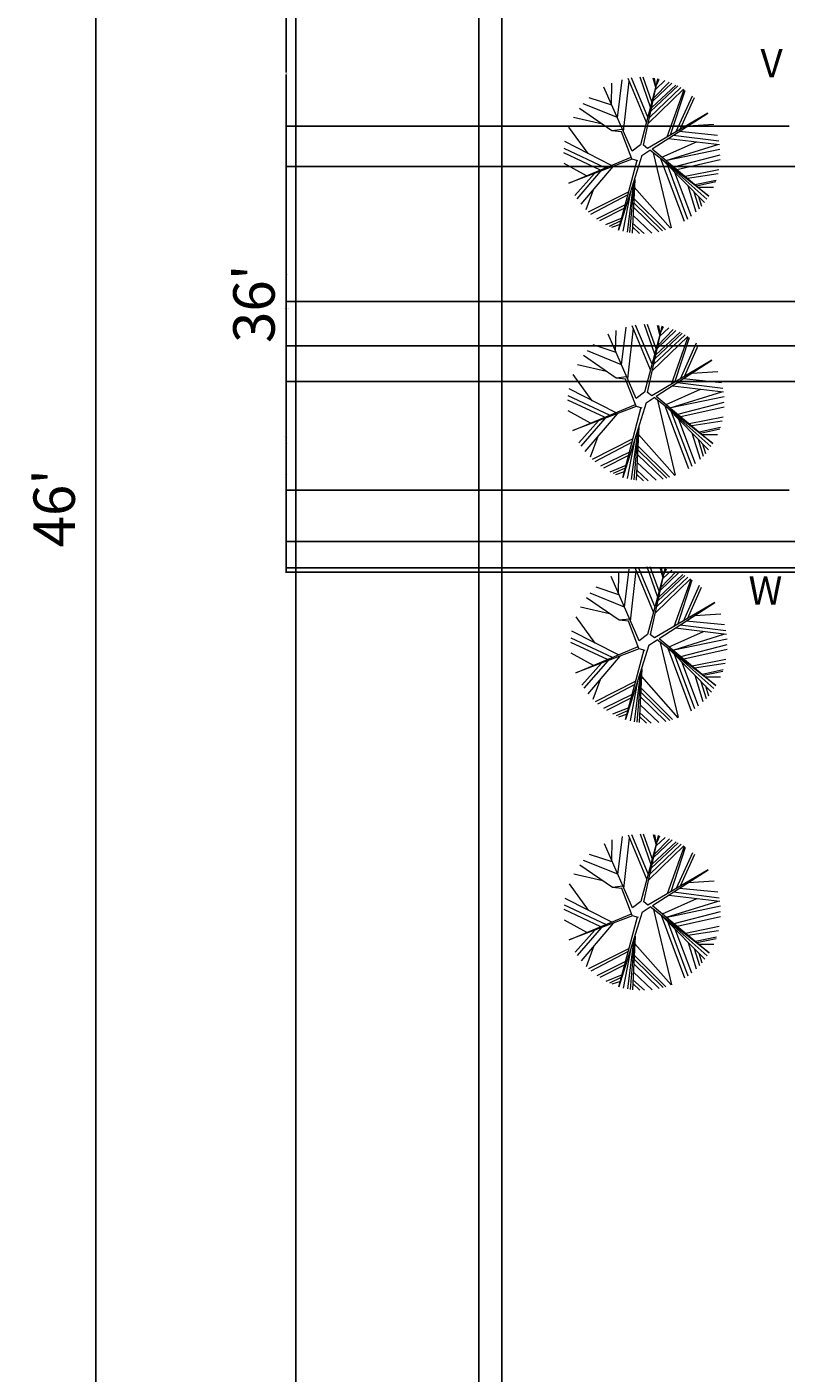
# Model space of a CAD drawing. Units: inches. Extents: x 503 to 1084, y -605 to 132.
# Tile 2 of 14: x 503 to 649, y -437 to -177. Entities that reach past the tile are written whole.
import ezdxf

# ---------------------------------------------------------------- set-up
doc = ezdxf.new("R2010")
doc.units = ezdxf.units.IN
doc.header["$MEASUREMENT"] = 0
for name, color, linetype, lineweight in [('A-ANNO-DIMS', 7, 'Continuous', 18), ('A-ANNO-TEXT', 7, 'Continuous', 18), ('C-PROP', 1, 'Continuous', 25)]:
    doc.layers.add(name, color=color, linetype=linetype, lineweight=lineweight)
doc.layers.add('GRASS', color=90, linetype='Continuous', lineweight=13, transparency=0.7)
doc.styles.get("Standard").update_dxf_attribs({"font": 'arial.ttf'})
doc.dimstyles.get("Standard").update_dxf_attribs({"dimtxt": 0.18, "dimasz": 0.18, "dimexe": 0.18, "dimexo": 0.0625, "dimgap": 0.09, "dimtad": 0, "dimtih": 1, "dimtoh": 1, "dimdec": 1, "dimzin": 0, "dimdsep": 46, "dimlunit": 4, "dimtxsty": 'Standard', "dimcen": 0.09, "dimadec": 0, "dimazin": 0, "dimtfac": 1, "dimtdec": 1, "dimtofl": 0, "dimtmove": 0, "dimatfit": 3, "dimfxl": 1, "dimtolj": 1, "dimtzin": 0, "dimarcsym": 0})

# ---------------------------------------------------------------- blocks, each defined once
blk = doc.blocks.new('A$C4FA53466')
at = {"color": 0}
for p, q in [((0.501, 1.356), (0.505, 1.578)), ((0.563, 1.216), (0.612, 1.614)), ((0.627, 1.07), (0.687, 1.601)), ((0.867, 1.166), (0.675, 1.628)), ((0.882, 1.223), (0.709, 1.633)), ((0.91, 1.328), (0.802, 1.64)), ((0.988, 1.623), (0.804, 0.931)), ((0.925, 1.384), (0.834, 1.64)), ((0.836, 0.927), (0.988, 1.623)), ((0.922, 1.323), (1.176, 1.559)), ((0.964, 1.534), (0.938, 1.632)), ((0.938, 1.393), (1.132, 1.579)), ((0.945, 1.425), (1.104, 1.59)), ((0.967, 1.545), (0.952, 1.63)), ((0.965, 1.517), (1.059, 1.605)), ((0.974, 1.559), (1.002, 1.62)), ((0.505, 1.347), (0.266, 1.426)), ((0.717, 0.864), (0.422, 1.538)), ((0.887, 1.159), (1.256, 1.515)), ((0.901, 1.223), (1.228, 1.532)), ((0.914, 1.283), (1.197, 1.549)), ((1.085, 1.015), (1.262, 1.512)), ((1.121, 1.036), (1.274, 1.503)), ((1.18, 1.071), (1.349, 1.447)), ((1.222, 1.096), (1.37, 1.428)), ((0.506, 1.079), (0.165, 1.314)), ((0.562, 1.217), (0.205, 1.363)), ((0.406, 1.148), (0.102, 1.217)), ((1.509, 1.265), (0.879, 0.894)), ((0.926, 0.889), (1.509, 1.265)), ((1.3, 1.13), (1.573, 1.147)), ((0.255, 0.841), (0.055, 1.116)), ((0.614, 1.092), (0.506, 1.079)), ((0.604, 1.069), (0.506, 1.079)), ((0.715, 0.784), (0.604, 1.069)), ((1.097, 0.999), (1.632, 0.934)), ((1.148, 1.032), (1.626, 0.972)), ((1.211, 1.073), (1.612, 1.034)), ((0.384, 0.667), (0, 0.848)), ((0.436, 0.689), (0.003, 0.892)), ((0.501, 0.716), (0.012, 0.965)), ((0.804, 0.931), (0.717, 0.864)), ((0.82, 0.82), (0.904, 0.875)), ((0.879, 0.894), (0.836, 0.927)), ((1.521, 0.394), (0.904, 0.875)), ((0.926, 0.889), (1.521, 0.394)), ((0.938, 0.848), (1.126, 0.059)), ((1.03, 0.802), (1.392, 0.963)), ((1.073, 0.767), (1.614, 0.936)), ((1.081, 0.769), (1.638, 0.886)), ((0.237, 0.605), (0.004, 0.735)), ((0.053, 0.528), (0.708, 0.803)), ((0.716, 0.781), (0.053, 0.528)), ((0.82, 0.82), (0.575, 0.037)), ((0.575, 0.037), (0.769, 0.772)), ((0.715, 0.784), (0.775, 0.767)), ((1.016, 0.788), (1.263, 0.13)), ((1.04, 0.769), (1.475, 0.326)), ((1.06, 0.754), (1.5, 0.362)), ((1.083, 0.725), (1.298, 0.153)), ((1.153, 0.701), (1.64, 0.826)), ((1.185, 0.674), (1.639, 0.776)), ((0.321, 0.63), (0.115, 0.4)), ((0.387, 0.655), (0.137, 0.366)), ((0.516, 0.704), (0.179, 0.309)), ((0.744, 0.569), (0.717, 0.006)), ((1.161, 0.646), (1.335, 0.182)), ((1.273, 0.601), (1.627, 0.672)), ((1.298, 0.58), (1.618, 0.629)), ((0.313, 0.466), (0.232, 0.248)), ((0.682, 0.44), (0.255, 0.225)), ((0.701, 0.44), (0.621, 0.024)), ((0.732, 0.539), (0.664, 0.015)), ((0.737, 0.554), (0.691, 0.01)), ((0.74, 0.488), (1.121, 0.057)), ((1.301, 0.503), (1.386, 0.227)), ((1.365, 0.438), (1.42, 0.26)), ((1.376, 0.515), (1.599, 0.562)), ((1.392, 0.502), (1.593, 0.545)), ((1.412, 0.486), (1.569, 0.486)), ((0.673, 0.407), (0.281, 0.201)), ((0.645, 0.301), (0.342, 0.153)), ((0.733, 0.326), (1.037, 0.029)), ((0.735, 0.369), (1.067, 0.038)), ((1.413, 0.39), (1.444, 0.288)), ((0.636, 0.267), (0.375, 0.133)), ((0.608, 0.161), (0.439, 0.093)), ((0.726, 0.192), (0.924, 0.006)), ((0.73, 0.277), (0.998, 0.019)), ((0.6, 0.133), (0.475, 0.076)), ((0.59, 0.094), (0.501, 0.064)), ((0.72, 0.07), (0.793, 0)), ((0.722, 0.111), (0.842, 0))]:
    blk.add_line(p, q, dxfattribs=at)
blk = doc.blocks.new('_ArchTick')
at = {"color": 0, "linetype": 'ByBlock', "const_width": 0.15}
blk.add_lwpolyline([(-0.5, -0.5), (0.5, 0.5)], dxfattribs=at)
blk = doc.blocks.new('_Oblique')
at = {"color": 0, "linetype": 'ByBlock', "lineweight": -2}
blk.add_line((-0.5, -0.5), (0.5, 0.5), dxfattribs=at)
blk = doc.blocks.new('*D10')
at = {"layer": 'A-ANNO-DIMS', "color": 0, "lineweight": -2, "transparency": 16777216}
blk.add_line((516.2, 6.18), (516.2, -545.82), dxfattribs=at)
at = {"layer": 'Defpoints', "color": 0, "transparency": 16777216}
for p in [(590.09, 6.18), (516.2, -545.82), (590.09, -545.82)]:
    blk.add_point(p, dxfattribs=at)
at = {"layer": 'A-ANNO-DIMS', "color": 0, "lineweight": -2, "transparency": 16777216, "xscale": 5, "yscale": 5, "zscale": 5}
for name, p, rotation in [('_ArchTick', (516.2, 6.18), 90), ('_Oblique', (516.2, -545.82), 270)]:
    blk.add_blockref(name, p, dxfattribs=dict(at, rotation=rotation))
at = {"layer": 'A-ANNO-DIMS', "color": 0, "transparency": 16777216, "insert": (508.12, -269.82), "char_height": 8, "attachment_point": 5, "rotation": 90}
blk.add_mtext("\\A1;46'", dxfattribs=at)
blk = doc.blocks.new('*D12')
at = {"layer": 'A-ANNO-DIMS', "color": 0, "lineweight": -2, "transparency": 16777216}
blk.add_line((554.79, -17.82), (554.79, -442.82), dxfattribs=at)
at = {"layer": 'Defpoints', "color": 0, "transparency": 16777216}
for p in [(650.09, -17.82), (554.79, -442.82), (650.09, -442.82)]:
    blk.add_point(p, dxfattribs=at)
at = {"layer": 'A-ANNO-DIMS', "color": 0, "lineweight": -2, "transparency": 16777216, "xscale": 5, "yscale": 5, "zscale": 5}
for name, p, rotation in [('_ArchTick', (554.79, -17.82), 90), ('_Oblique', (554.79, -442.82), 270)]:
    blk.add_blockref(name, p, dxfattribs=dict(at, rotation=rotation))
at = {"layer": 'A-ANNO-DIMS', "color": 0, "transparency": 16777216, "insert": (546.7, -230.32), "char_height": 8, "attachment_point": 5, "rotation": 90}
blk.add_mtext("\\A1;36'", dxfattribs=at)
blk = doc.blocks.new('*D54')
at = {"layer": 'A-ANNO-DIMS', "color": 0, "lineweight": -2, "transparency": 16777216}
for p, q in [((650.03, -195.98), (552.76, -195.98)), ((552.94, -196.16), (552.94, -230.97)), ((552.94, -266.14), (552.94, -231.33)), ((650.03, -266.32), (552.76, -266.32))]:
    blk.add_line(p, q, dxfattribs=at)
at = {"layer": 'A-ANNO-DIMS', "color": 0, "transparency": 16777216}
for points in [[(552.91, -196.16), (552.97, -196.16), (552.94, -195.98)], [(552.91, -266.14), (552.97, -266.14), (552.94, -266.32)]]:
    blk.add_solid(points, dxfattribs=at)
at = {"layer": 'Defpoints', "color": 0, "transparency": 16777216}
for p in [(650.09, -195.98), (552.94, -266.32), (650.09, -266.32)]:
    blk.add_point(p, dxfattribs=at)
at = {"layer": 'A-ANNO-DIMS', "color": 0, "transparency": 16777216, "insert": (552.94, -231.15), "char_height": 0.18, "attachment_point": 5}
blk.add_mtext('\\A1;5\'-10 1/2"', dxfattribs=at)
blk = doc.blocks.new('*D55')
at = {"layer": 'A-ANNO-DIMS', "color": 0, "lineweight": -2, "transparency": 16777216}
for p, q in [((779.03, -245.32), (552.76, -245.32)), ((552.94, -245.5), (552.94, -263.13)), ((552.94, -281.14), (552.94, -263.5)), ((779.03, -281.32), (552.76, -281.32))]:
    blk.add_line(p, q, dxfattribs=at)
at = {"layer": 'A-ANNO-DIMS', "color": 0, "transparency": 16777216}
for points in [[(552.91, -245.5), (552.97, -245.5), (552.94, -245.32)], [(552.91, -281.14), (552.97, -281.14), (552.94, -281.32)]]:
    blk.add_solid(points, dxfattribs=at)
at = {"layer": 'Defpoints', "color": 0, "transparency": 16777216}
for p in [(779.09, -245.32), (552.94, -281.32), (779.09, -281.32)]:
    blk.add_point(p, dxfattribs=at)
at = {"layer": 'A-ANNO-DIMS', "color": 0, "transparency": 16777216, "insert": (552.94, -263.32), "char_height": 0.18, "attachment_point": 5}
blk.add_mtext('\\A1;3\'-0"', dxfattribs=at)
blk = doc.blocks.new('*D56')
at = {"layer": 'A-ANNO-DIMS', "color": 0, "lineweight": -2, "transparency": 16777216}
for p, q in [((779.03, -167.82), (552.76, -167.82)), ((552.94, -168), (552.94, -185.63)), ((552.94, -203.64), (552.94, -186)), ((779.03, -203.82), (552.76, -203.82))]:
    blk.add_line(p, q, dxfattribs=at)
at = {"layer": 'A-ANNO-DIMS', "color": 0, "transparency": 16777216}
for points in [[(552.91, -168), (552.97, -168), (552.94, -167.82)], [(552.91, -203.64), (552.97, -203.64), (552.94, -203.82)]]:
    blk.add_solid(points, dxfattribs=at)
at = {"layer": 'Defpoints', "color": 0, "transparency": 16777216}
for p in [(779.09, -167.82), (552.94, -203.82), (779.09, -203.82)]:
    blk.add_point(p, dxfattribs=at)
at = {"layer": 'A-ANNO-DIMS', "color": 0, "transparency": 16777216, "insert": (552.94, -185.82), "char_height": 0.18, "attachment_point": 5}
blk.add_mtext('\\A1;3\'-0"', dxfattribs=at)
blk = doc.blocks.new('*D62')
at = {"layer": 'A-ANNO-DIMS', "color": 0, "lineweight": -2, "transparency": 16777216}
for p, q in [((779.03, -203.82), (552.76, -203.82)), ((552.94, -204), (552.94, -224.38)), ((552.94, -245.14), (552.94, -224.75)), ((779.03, -245.32), (552.76, -245.32))]:
    blk.add_line(p, q, dxfattribs=at)
at = {"layer": 'A-ANNO-DIMS', "color": 0, "transparency": 16777216}
for points in [[(552.91, -204), (552.97, -204), (552.94, -203.82)], [(552.91, -245.14), (552.97, -245.14), (552.94, -245.32)]]:
    blk.add_solid(points, dxfattribs=at)
at = {"layer": 'Defpoints', "color": 0, "transparency": 16777216}
for p in [(779.09, -203.82), (552.94, -245.32), (779.09, -245.32)]:
    blk.add_point(p, dxfattribs=at)
at = {"layer": 'A-ANNO-DIMS', "color": 0, "transparency": 16777216, "insert": (552.94, -224.57), "char_height": 0.18, "attachment_point": 5}
blk.add_mtext('\\A1;3\'-5 1/2"', dxfattribs=at)
blk = doc.blocks.new('*D72')
at = {"layer": 'A-ANNO-DIMS', "color": 0, "lineweight": -2, "transparency": 16777216}
for p, q in [((948.89, -229.87), (552.76, -229.87)), ((552.94, -230.05), (552.94, -255.86)), ((552.94, -282.03), (552.94, -256.22)), ((949.25, -282.21), (552.76, -282.21))]:
    blk.add_line(p, q, dxfattribs=at)
at = {"layer": 'A-ANNO-DIMS', "color": 0, "transparency": 16777216}
for points in [[(552.91, -230.05), (552.97, -230.05), (552.94, -229.87)], [(552.91, -282.03), (552.97, -282.03), (552.94, -282.21)]]:
    blk.add_solid(points, dxfattribs=at)
at = {"layer": 'Defpoints', "color": 0, "transparency": 16777216}
for p in [(948.95, -229.87), (552.94, -282.21), (949.31, -282.21)]:
    blk.add_point(p, dxfattribs=at)
at = {"layer": 'A-ANNO-DIMS', "color": 0, "transparency": 16777216, "insert": (552.94, -256.04), "char_height": 0.18, "attachment_point": 5}
blk.add_mtext('\\A1;4\'-4 1/2"', dxfattribs=at)
blk = doc.blocks.new('*D77')
at = {"layer": 'A-ANNO-DIMS', "color": 0, "lineweight": -2, "transparency": 16777216}
for p, q in [((926.53, -238.47), (552.76, -238.47)), ((552.94, -238.65), (552.94, -257.17)), ((552.94, -276.07), (552.94, -257.54)), ((916.28, -276.25), (552.76, -276.25))]:
    blk.add_line(p, q, dxfattribs=at)
at = {"layer": 'A-ANNO-DIMS', "color": 0, "transparency": 16777216}
for points in [[(552.91, -238.65), (552.97, -238.65), (552.94, -238.47)], [(552.91, -276.07), (552.97, -276.07), (552.94, -276.25)]]:
    blk.add_solid(points, dxfattribs=at)
at = {"layer": 'Defpoints', "color": 0, "transparency": 16777216}
for p in [(926.59, -238.47), (552.94, -276.25), (916.35, -276.25)]:
    blk.add_point(p, dxfattribs=at)
at = {"layer": 'A-ANNO-DIMS', "color": 0, "transparency": 16777216, "insert": (552.94, -257.36), "char_height": 0.18, "attachment_point": 5}
blk.add_mtext('\\A1;3\'-2"', dxfattribs=at)

msp = doc.modelspace()

# ---------------------------------------------------------------- linework, layer by layer
at = {"layer": 'C-PROP'}
for p, q in [((590.09, 6.18), (590.09, -545.82)), ((594.59, -541.32), (594.59, 1.68))]:
    msp.add_line(p, q, dxfattribs=at)

# ---------------------------------------------------------------- block references
at = {"layer": 'GRASS', "xscale": 18.41745235960633, "yscale": 18.41745235960633, "zscale": 18.41745235960633}
for p in [(606.51, -216.77), (607.31, -264.55), (607.87, -311.36), (606.58, -362.98)]:
    msp.add_blockref('A$C4FA53466', p, dxfattribs=at)

# ---------------------------------------------------------------- texts
at = {"layer": 'A-ANNO-TEXT'}
for s, p in [('V', (644.51, -186.57)), ('W', (642.19, -288.44))]:
    msp.add_text(s, height=5.44, dxfattribs=at).set_placement(p)

# ---------------------------------------------------------------- dimensions: what is measured, and where the dimension line sits
at = {"layer": 'A-ANNO-DIMS'}
for base, p1, p2, override, picture, middle in [((516.2, -545.82), (590.09, 6.18), (590.09, -545.82), {"dimtxt": 8, "dimasz": 5, "dimgap": 4, "dimtad": 1, "dimtih": 0, "dimblk1": 'ArchTick', "dimblk2": 'Oblique', "dimsah": 1, "dimse1": 1, "dimse2": 1, "dimclrd": 0, "dimclre": 0, "dimclrt": 0}, '*D10', (508.12, -269.82)), ((552.94, -203.82), (779.09, -167.82), (779.09, -203.82), {"dimdec": 1, "dimlfac": 1, "dimrnd": 0, "dimzin": 1, "dimdsep": 46, "dimlunit": 4, "dimfrac": 2}, '*D56', (552.94, -185.82)), ((552.94, -266.32), (650.09, -195.98), (650.09, -266.32), {"dimdec": 1, "dimlfac": 1, "dimrnd": 0, "dimzin": 1, "dimdsep": 46, "dimlunit": 4, "dimfrac": 2}, '*D54', (552.94, -231.15)), ((552.94, -245.32), (779.09, -203.82), (779.09, -245.32), {"dimdec": 1, "dimlfac": 1, "dimrnd": 0, "dimzin": 1, "dimdsep": 46, "dimlunit": 4, "dimfrac": 2}, '*D62', (552.94, -224.57)), ((552.94, -282.21), (948.95, -229.87), (949.31, -282.21), {"dimdec": 1, "dimlfac": 1, "dimrnd": 0, "dimzin": 1, "dimdsep": 46, "dimlunit": 4, "dimfrac": 2}, '*D72', (552.94, -256.04)), ((552.94, -276.25), (926.59, -238.47), (916.35, -276.25), {"dimdec": 1, "dimlfac": 1, "dimrnd": 0, "dimzin": 1, "dimdsep": 46, "dimlunit": 4, "dimfrac": 2}, '*D77', (552.94, -257.36)), ((552.94, -281.32), (779.09, -245.32), (779.09, -281.32), {"dimdec": 1, "dimlfac": 1, "dimrnd": 0, "dimzin": 1, "dimdsep": 46, "dimlunit": 4, "dimfrac": 2}, '*D55', (552.94, -263.32))]:
    dim = msp.add_linear_dim(base=base, p1=p1, p2=p2, angle=90, dimstyle='Standard', override=override, dxfattribs=at)
    dim.commit()
    dim.dimension.update_dxf_attribs({"geometry": picture, "text_midpoint": middle})
dim = msp.add_linear_dim(base=(554.79, -442.82), p1=(650.09, -17.82), p2=(650.09, -442.82), angle=90, text="36'", dimstyle='Standard', override={"dimtxt": 8, "dimasz": 5, "dimgap": 4, "dimtad": 1, "dimtih": 0, "dimblk1": 'ArchTick', "dimblk2": 'Oblique', "dimsah": 1, "dimse1": 1, "dimse2": 1, "dimclrd": 0, "dimclre": 0, "dimclrt": 0}, dxfattribs=at)
dim.commit()
dim.dimension.update_dxf_attribs({"geometry": '*D12', "text_midpoint": (546.7, -230.32)})

doc.saveas('drawing.dxf')
